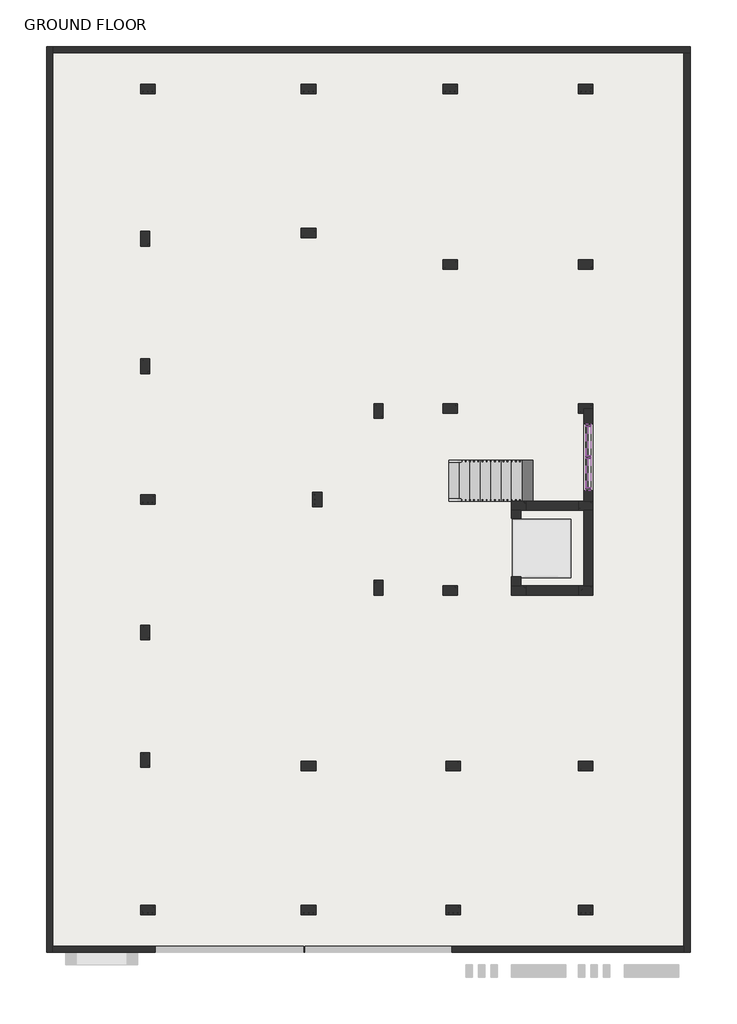
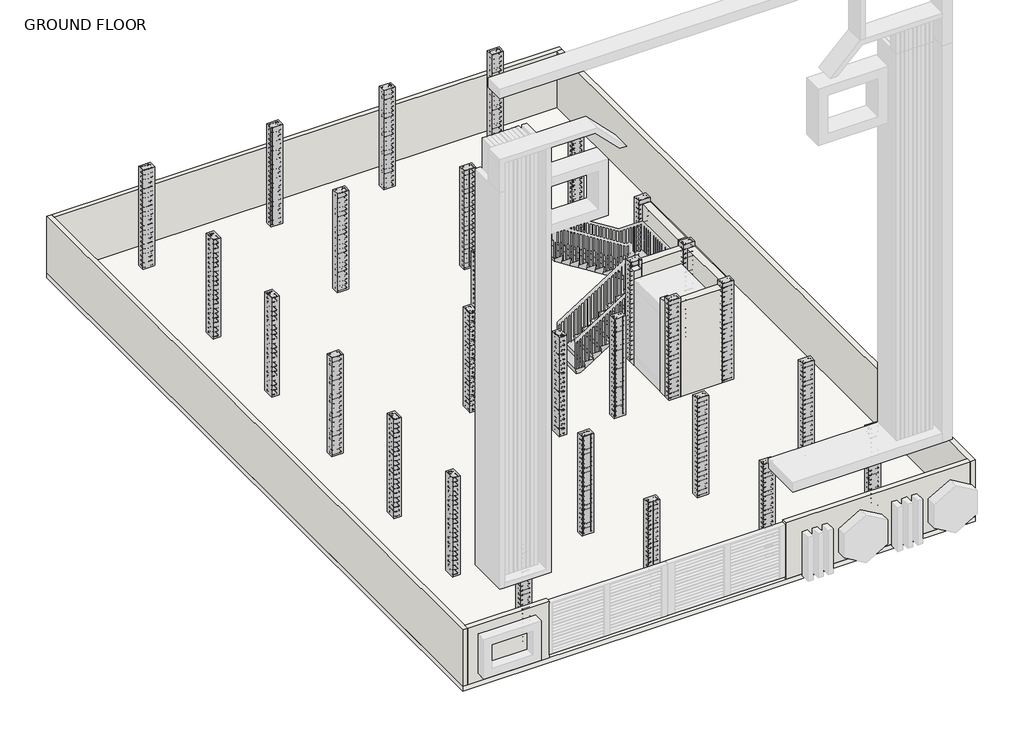
# One storey, part 1 of 7: 29 columns, 12 members, 12 walls, 4 plates, 1 slab, 1 stair flight.
"""IFC4 building model written with IfcOpenShell, lengths in millimetres."""

from ifc_helpers import new_model, si_unit, frame, origin, origin_with_axes, place, context, project, spatial, polyline, outline, extrude, faceted_brep, transform, mapped, element, save
from components import column_add0f710, member_7007ad49, member_abeaf8ac, member_a715cb85, member_410c6227, member_c4de40ee, member_73c23c35, system_panel_glazed_a527b3ca, system_panel_glazed_0825baf2

model = new_model("IFC4")

# Units and contexts
model_context = context("Model", 3, world=origin())
ifc_project = project(units=[si_unit("LENGTHUNIT", "METRE", prefix="MILLI")], contexts=[model_context])

# Site, building, storey
site = spatial("IfcSite", under=ifc_project)
building = spatial("IfcBuilding", under=site)
storey = spatial("IfcBuildingStorey", under=building, Name="GROUND FLOOR", Elevation=0.0)

# Columns
placement = place(None, origin())
column_shape = column_add0f710(model_context)
element("IfcColumn", 1, ObjectType="Concrete-Rectangular-Column : 1'2\"X9\"", at=placement, inside=storey, context=model_context, shape_type="MappedRepresentation", body=[
    mapped(column_shape, transform((-6074.3833787, 10029.759934, 0.0), x_axis=(0.0, 1.0, 0.0), y_axis=(-1.0, 0.0, 0.0), z_axis=(0.0, 0.0, 1.0))),
])
element("IfcColumn", 2, ObjectType="Concrete-Rectangular-Column : 1'2\"X9\"", at=placement, inside=storey, context=model_context, shape_type="MappedRepresentation", body=[
    mapped(column_shape, transform((-2162.7833787, 10029.759934, 0.0), x_axis=(0.0, 1.0, 0.0), y_axis=(-1.0, 0.0, 0.0), z_axis=(0.0, 0.0, 1.0))),
])
element("IfcColumn", 3, ObjectType="Concrete-Rectangular-Column : 1'2\"X9\"", at=placement, inside=storey, context=model_context, shape_type="MappedRepresentation", body=[
    mapped(column_shape, transform((1278.9166213, 10029.759934, 0.0), x_axis=(0.0, 1.0, 0.0), y_axis=(-1.0, 0.0, 0.0), z_axis=(0.0, 0.0, 1.0))),
])
element("IfcColumn", 4, ObjectType="Concrete-Rectangular-Column : 1'2\"X9\"", at=placement, inside=storey, context=model_context, shape_type="MappedRepresentation", body=[
    mapped(column_shape, transform((4580.9166213, 10029.759934, 0.0), x_axis=(0.0, 1.0, 0.0), y_axis=(-1.0, 0.0, 0.0), z_axis=(0.0, 0.0, 1.0))),
])
element("IfcColumn", 5, ObjectType="Concrete-Rectangular-Column : 1'2\"X9\"", at=placement, inside=storey, context=model_context, shape_type="MappedRepresentation", body=[
    mapped(column_shape, transform((4580.9166213, 5762.559934, 0.0), x_axis=(0.0, 1.0, 0.0), y_axis=(-1.0, 0.0, 0.0), z_axis=(0.0, 0.0, 1.0))),
])
element("IfcColumn", 6, ObjectType="Concrete-Rectangular-Column : 1'2\"X9\"", at=placement, inside=storey, context=model_context, shape_type="MappedRepresentation", body=[
    mapped(column_shape, transform((1278.9166213, 5762.559934, 0.0), x_axis=(0.0, 1.0, 0.0), y_axis=(-1.0, 0.0, 0.0), z_axis=(0.0, 0.0, 1.0))),
])
element("IfcColumn", 7, ObjectType="Concrete-Rectangular-Column : 1'2\"X9\"", at=placement, inside=storey, context=model_context, shape_type="MappedRepresentation", body=[
    mapped(column_shape, transform((-2162.7833787, 6524.559934, 0.0), x_axis=(0.0, 1.0, 0.0), y_axis=(-1.0, 0.0, 0.0), z_axis=(0.0, 0.0, 1.0))),
])
element("IfcColumn", 8, ObjectType="Concrete-Rectangular-Column : 1'2\"X9\"", at=placement, inside=storey, context=model_context, shape_type="MappedRepresentation", body=[
    mapped(column_shape, transform((-6137.8833787, 6384.859934, 0.0), x_axis=(-1.0, 0.0, 0.0), y_axis=(0.0, -1.0, 0.0), z_axis=(0.0, 0.0, 1.0))),
])
element("IfcColumn", 9, ObjectType="Concrete-Rectangular-Column : 1'2\"X9\"", at=placement, inside=storey, context=model_context, shape_type="MappedRepresentation", body=[
    mapped(column_shape, transform((-6137.8833787, 3286.059934, 0.0), x_axis=(-1.0, 0.0, 0.0), y_axis=(0.0, -1.0, 0.0), z_axis=(0.0, 0.0, 1.0))),
])
element("IfcColumn", 10, ObjectType="Concrete-Rectangular-Column : 1'2\"X9\"", at=placement, inside=storey, context=model_context, shape_type="MappedRepresentation", body=[
    mapped(column_shape, transform((-460.9833787, 2193.859934, 0.0), x_axis=(-1.0, 0.0, 0.0), y_axis=(0.0, -1.0, 0.0), z_axis=(0.0, 0.0, 1.0))),
])
element("IfcColumn", 11, ObjectType="Concrete-Rectangular-Column : 1'2\"X9\"", at=placement, inside=storey, context=model_context, shape_type="MappedRepresentation", body=[
    mapped(column_shape, transform((1278.9166213, 2257.359934, 0.0), x_axis=(0.0, -1.0, 0.0), y_axis=(1.0, 0.0, 0.0), z_axis=(0.0, 0.0, 1.0))),
])
element("IfcColumn", 12, ObjectType="Concrete-Rectangular-Column : 1'2\"X9\"", at=placement, inside=storey, context=model_context, shape_type="MappedRepresentation", body=[
    mapped(column_shape, transform((4580.9166213, 2257.359934, 0.0), x_axis=(0.0, -1.0, 0.0), y_axis=(1.0, 0.0, 0.0), z_axis=(0.0, 0.0, 1.0))),
])
element("IfcColumn", 13, ObjectType="Concrete-Rectangular-Column : 1'2\"X9\"", at=placement, inside=storey, context=model_context, shape_type="MappedRepresentation", body=[
    mapped(column_shape, transform((4580.9166213, -104.840066, 0.0), x_axis=(0.0, -1.0, 0.0), y_axis=(1.0, 0.0, 0.0), z_axis=(0.0, 0.0, 1.0))),
])
element("IfcColumn", 14, ObjectType="Concrete-Rectangular-Column : 1'2\"X9\"", at=placement, inside=storey, context=model_context, shape_type="MappedRepresentation", body=[
    mapped(column_shape, transform((2955.3166213, -104.840066, 0.0), x_axis=(0.0, -1.0, 0.0), y_axis=(1.0, 0.0, 0.0), z_axis=(0.0, 0.0, 1.0))),
])
element("IfcColumn", 15, ObjectType="Concrete-Rectangular-Column : 1'2\"X9\"", at=placement, inside=storey, context=model_context, shape_type="MappedRepresentation", body=[
    mapped(column_shape, transform((-1946.8833787, 47.559934, 0.0), x_axis=(1.0, 0.0, 0.0), y_axis=(0.0, 1.0, 0.0), z_axis=(0.0, 0.0, 1.0))),
])
element("IfcColumn", 16, ObjectType="Concrete-Rectangular-Column : 1'2\"X9\"", at=placement, inside=storey, context=model_context, shape_type="MappedRepresentation", body=[
    mapped(column_shape, transform((-6074.3833787, 47.559934, 0.0), x_axis=(0.0, 1.0, 0.0), y_axis=(-1.0, 0.0, 0.0), z_axis=(0.0, 0.0, 1.0))),
])
element("IfcColumn", 17, ObjectType="Concrete-Rectangular-Column : 1'2\"X9\"", at=placement, inside=storey, context=model_context, shape_type="MappedRepresentation", body=[
    mapped(column_shape, transform((-6137.8833787, -3190.940066, 0.0), x_axis=(-1.0, 0.0, 0.0), y_axis=(0.0, -1.0, 0.0), z_axis=(0.0, 0.0, 1.0))),
])
element("IfcColumn", 18, ObjectType="Concrete-Rectangular-Column : 1'2\"X9\"", at=placement, inside=storey, context=model_context, shape_type="MappedRepresentation", body=[
    mapped(column_shape, transform((-6137.8833787, -6289.740066, 0.0), x_axis=(-1.0, 0.0, 0.0), y_axis=(0.0, -1.0, 0.0), z_axis=(0.0, 0.0, 1.0))),
])
element("IfcColumn", 19, ObjectType="Concrete-Rectangular-Column : 1'2\"X9\"", at=placement, inside=storey, context=model_context, shape_type="MappedRepresentation", body=[
    mapped(column_shape, transform((-2162.7833787, -6429.440066, 0.0), x_axis=(0.0, -1.0, 0.0), y_axis=(1.0, 0.0, 0.0), z_axis=(0.0, 0.0, 1.0))),
])
element("IfcColumn", 20, ObjectType="Concrete-Rectangular-Column : 1'2\"X9\"", at=placement, inside=storey, context=model_context, shape_type="MappedRepresentation", body=[
    mapped(column_shape, transform((-6074.3833787, -9934.640066, 0.0), x_axis=(0.0, -1.0, 0.0), y_axis=(1.0, 0.0, 0.0), z_axis=(0.0, 0.0, 1.0))),
])
element("IfcColumn", 21, ObjectType="Concrete-Rectangular-Column : 1'2\"X9\"", at=placement, inside=storey, context=model_context, shape_type="MappedRepresentation", body=[
    mapped(column_shape, transform((-2162.7833787, -9934.640066, 0.0), x_axis=(0.0, -1.0, 0.0), y_axis=(1.0, 0.0, 0.0), z_axis=(0.0, 0.0, 1.0))),
])
element("IfcColumn", 22, ObjectType="Concrete-Rectangular-Column : 1'2\"X9\"", at=placement, inside=storey, context=model_context, shape_type="MappedRepresentation", body=[
    mapped(column_shape, transform((1355.1166213, -9934.640066, 0.0), x_axis=(0.0, -1.0, 0.0), y_axis=(1.0, 0.0, 0.0), z_axis=(0.0, 0.0, 1.0))),
])
element("IfcColumn", 23, ObjectType="Concrete-Rectangular-Column : 1'2\"X9\"", at=placement, inside=storey, context=model_context, shape_type="MappedRepresentation", body=[
    mapped(column_shape, transform((4580.9166213, -9934.640066, 0.0), x_axis=(0.0, -1.0, 0.0), y_axis=(1.0, 0.0, 0.0), z_axis=(0.0, 0.0, 1.0))),
])
element("IfcColumn", 24, ObjectType="Concrete-Rectangular-Column : 1'2\"X9\"", at=placement, inside=storey, context=model_context, shape_type="MappedRepresentation", body=[
    mapped(column_shape, transform((4580.9166213, -6429.440066, 0.0), x_axis=(0.0, -1.0, 0.0), y_axis=(1.0, 0.0, 0.0), z_axis=(0.0, 0.0, 1.0))),
])
element("IfcColumn", 25, ObjectType="Concrete-Rectangular-Column : 1'2\"X9\"", at=placement, inside=storey, context=model_context, shape_type="MappedRepresentation", body=[
    mapped(column_shape, transform((1355.1166213, -6429.440066, 0.0), x_axis=(0.0, -1.0, 0.0), y_axis=(1.0, 0.0, 0.0), z_axis=(0.0, 0.0, 1.0))),
])
element("IfcColumn", 26, ObjectType="Concrete-Rectangular-Column : 1'2\"X9\"", at=placement, inside=storey, context=model_context, shape_type="MappedRepresentation", body=[
    mapped(column_shape, transform((1278.9166213, -2162.240066, 0.0), x_axis=(0.0, -1.0, 0.0), y_axis=(1.0, 0.0, 0.0), z_axis=(0.0, 0.0, 1.0))),
])
element("IfcColumn", 27, ObjectType="Concrete-Rectangular-Column : 1'2\"X9\"", at=placement, inside=storey, context=model_context, shape_type="MappedRepresentation", body=[
    mapped(column_shape, transform((2955.3166213, -2162.240066, 0.0), x_axis=(0.0, -1.0, 0.0), y_axis=(1.0, 0.0, 0.0), z_axis=(0.0, 0.0, 1.0))),
])
element("IfcColumn", 28, ObjectType="Concrete-Rectangular-Column : 1'2\"X9\"", at=placement, inside=storey, context=model_context, shape_type="MappedRepresentation", body=[
    mapped(column_shape, transform((4580.9166213, -2162.240066, 0.0), x_axis=(0.0, -1.0, 0.0), y_axis=(1.0, 0.0, 0.0), z_axis=(0.0, 0.0, 1.0))),
])
element("IfcColumn", 29, ObjectType="Concrete-Rectangular-Column : 1'2\"X9\"", at=placement, inside=storey, context=model_context, shape_type="MappedRepresentation", body=[
    mapped(column_shape, transform((-460.9833787, -2098.740066, 0.0), x_axis=(1.0, 0.0, 0.0), y_axis=(0.0, 1.0, 0.0), z_axis=(0.0, 0.0, 1.0))),
])

# Members
member_shape = member_7007ad49(model_context)
element("IfcMember", 30, ObjectType="Rectangular Mullion : 2.5\" x 5\" rectangular", at=placement, inside=storey, context=model_context, shape_type="MappedRepresentation", body=[
    mapped(member_shape, transform((4644.4166213, 1825.559934, 2438.4), x_axis=(0.0, 0.0, 1.0), y_axis=(1.0, 0.0, 0.0), z_axis=(0.0, 1.0, 0.0))),
])
element("IfcMember", 31, ObjectType="Rectangular Mullion : 2.5\" x 5\" rectangular", at=placement, inside=storey, context=model_context, shape_type="MappedRepresentation", body=[
    mapped(member_shape, transform((4644.4166213, 1044.509934, 2438.4), x_axis=(0.0, 0.0, 1.0), y_axis=(1.0, 0.0, 0.0), z_axis=(0.0, 1.0, 0.0))),
])
element("IfcMember", 32, ObjectType="Rectangular Mullion : 2.5\" x 5\" rectangular", at=placement, inside=storey, context=model_context, shape_type="MappedRepresentation", body=[
    mapped(member_shape, transform((4644.4166213, 326.959934, 457.2), x_axis=(0.0, 0.0, -1.0), y_axis=(1.0, 0.0, 0.0), z_axis=(0.0, -1.0, 0.0))),
])
element("IfcMember", 33, ObjectType="Rectangular Mullion : 2.5\" x 5\" rectangular", at=placement, inside=storey, context=model_context, shape_type="MappedRepresentation", body=[
    mapped(member_shape, transform((4644.4166213, 1108.009934, 457.2), x_axis=(0.0, 0.0, -1.0), y_axis=(1.0, 0.0, 0.0), z_axis=(0.0, -1.0, 0.0))),
])
member_2_shape = member_abeaf8ac(model_context)
element("IfcMember", 34, ObjectType="Rectangular Mullion : 2.5\" x 5\" rectangular", at=placement, inside=storey, context=model_context, shape_type="MappedRepresentation", body=[
    mapped(member_2_shape, transform((4644.4166213, 1044.509934, 1524.0), x_axis=(0.0, 0.0, 1.0), y_axis=(1.0, 0.0, 0.0), z_axis=(0.0, 1.0, 0.0))),
])
element("IfcMember", 35, ObjectType="Rectangular Mullion : 2.5\" x 5\" rectangular", at=placement, inside=storey, context=model_context, shape_type="MappedRepresentation", body=[
    mapped(member_2_shape, transform((4644.4166213, 1825.559934, 1524.0), x_axis=(0.0, 0.0, 1.0), y_axis=(1.0, 0.0, 0.0), z_axis=(0.0, 1.0, 0.0))),
])
member_3_shape = member_a715cb85(model_context)
element("IfcMember", 36, ObjectType="Rectangular Mullion : 2.5\" x 5\" rectangular", at=placement, inside=storey, context=model_context, shape_type="MappedRepresentation", body=[
    mapped(member_3_shape, transform((4644.4166213, 1076.259934, 457.2), x_axis=(0.0, 1.0, 0.0), y_axis=(1.0, 0.0, 0.0), z_axis=(0.0, 0.0, -1.0))),
])
member_4_shape = member_410c6227(model_context)
element("IfcMember", 37, ObjectType="Rectangular Mullion : 2.5\" x 5\" rectangular", at=placement, inside=storey, context=model_context, shape_type="MappedRepresentation", body=[
    mapped(member_4_shape, transform((4644.4166213, 1076.259934, 1524.0), x_axis=(0.0, 1.0, 0.0), y_axis=(1.0, 0.0, 0.0), z_axis=(0.0, 0.0, -1.0))),
])
member_5_shape = member_c4de40ee(model_context)
element("IfcMember", 38, ObjectType="Rectangular Mullion : 2.5\" x 5\" rectangular", at=placement, inside=storey, context=model_context, shape_type="MappedRepresentation", body=[
    mapped(member_5_shape, transform((4644.4166213, 1889.059934, 457.2), x_axis=(0.0, 1.0, 0.0), y_axis=(1.0, 0.0, 0.0), z_axis=(0.0, 0.0, -1.0))),
])
member_6_shape = member_73c23c35(model_context)
element("IfcMember", 39, ObjectType="Rectangular Mullion : 2.5\" x 5\" rectangular", at=placement, inside=storey, context=model_context, shape_type="MappedRepresentation", body=[
    mapped(member_6_shape, transform((4644.4166213, 263.459934, 2438.4), x_axis=(0.0, -1.0, 0.0), y_axis=(1.0, 0.0, 0.0), z_axis=(0.0, 0.0, 1.0))),
])
element("IfcMember", 40, ObjectType="Rectangular Mullion : 2.5\" x 5\" rectangular", at=placement, inside=storey, context=model_context, shape_type="MappedRepresentation", body=[
    mapped(member_6_shape, transform((4644.4166213, 1889.059934, 1524.0), x_axis=(0.0, 1.0, 0.0), y_axis=(1.0, 0.0, 0.0), z_axis=(0.0, 0.0, -1.0))),
])
element("IfcMember", 41, ObjectType="Rectangular Mullion : 2.5\" x 5\" rectangular", at=placement, inside=storey, context=model_context, shape_type="MappedRepresentation", body=[
    mapped(member_5_shape, transform((4644.4166213, 263.459934, 1524.0), x_axis=(0.0, -1.0, 0.0), y_axis=(1.0, 0.0, 0.0), z_axis=(0.0, 0.0, 1.0))),
])

# Plates
system_panel_glazed_shape = system_panel_glazed_a527b3ca(model_context)
element("IfcPlate", 42, ObjectType="System Panel : Glazed", at=placement, inside=storey, context=model_context, shape_type="MappedRepresentation", body=[
    mapped(system_panel_glazed_shape, transform((4644.4166213, 685.734934, 520.7), x_axis=(0.0, 1.0, 0.0), y_axis=(-1.0, 0.0, 0.0), z_axis=(0.0, 0.0, 1.0))),
])
element("IfcPlate", 43, ObjectType="System Panel : Glazed", at=placement, inside=storey, context=model_context, shape_type="MappedRepresentation", body=[
    mapped(system_panel_glazed_shape, transform((4644.4166213, 1466.784934, 520.7), x_axis=(0.0, 1.0, 0.0), y_axis=(-1.0, 0.0, 0.0), z_axis=(0.0, 0.0, 1.0))),
])
system_panel_glazed_2_shape = system_panel_glazed_0825baf2(model_context)
element("IfcPlate", 44, ObjectType="System Panel : Glazed", at=placement, inside=storey, context=model_context, shape_type="MappedRepresentation", body=[
    mapped(system_panel_glazed_2_shape, transform((4644.4166213, 685.734934, 1555.75), x_axis=(0.0, 1.0, 0.0), y_axis=(-1.0, 0.0, 0.0), z_axis=(0.0, 0.0, 1.0))),
])
element("IfcPlate", 45, ObjectType="System Panel : Glazed", at=placement, inside=storey, context=model_context, shape_type="MappedRepresentation", body=[
    mapped(system_panel_glazed_2_shape, transform((4644.4166213, 1466.784934, 1555.75), x_axis=(0.0, 1.0, 0.0), y_axis=(-1.0, 0.0, 0.0), z_axis=(0.0, 0.0, 1.0))),
])

# Slab
element("IfcSlab", 46, ObjectType="6\"", at=placement, inside=storey, context=model_context, shape_type="SweptSolid", body=[
    extrude(outline(polyline([(7120.9166213, 11058.459934), (7120.9166213, -10963.340066), (-8538.1833787, -10963.340066), (-8538.1833787, 11058.459934), (7120.9166213, 11058.459934)])), frame((0.0, 0.0, -152.4), z_axis=(0.0, 0.0, 1.0), x_axis=(1.0, 0.0, 0.0)), (0.0, 0.0, 1.0), 152.4),
])

# Stair flight
element("IfcStairFlight", 47, ObjectType="3/4\" Nosing", at=placement, inside=storey, context=model_context, shape_type="Brep", body=[
    faceted_brep([(1253.5166213, 9.459934, 160.02), (1253.5166213, 1000.059934, 160.02), (1272.5666213, 1000.059934, 0.0), (1272.5666213, 9.459934, 0.0), (1526.5666213, 9.459934, 160.02), (1526.5666213, 1000.059934, 160.02), (1526.5666213, 1000.059934, 84.9690172), (1391.6951655, 1000.059934, 0.0), (1391.6951655, 9.459934, 0.0), (1526.5666213, 9.459934, 84.9690172), (1507.5166213, 1000.059934, 320.04), (1507.5166213, 9.459934, 320.04), (1780.5666213, 9.459934, 320.04), (1780.5666213, 1000.059934, 320.04), (1780.5666213, 1000.059934, 244.9890172), (1780.5666213, 9.459934, 244.9890172), (1761.5166213, 1000.059934, 480.06), (1761.5166213, 9.459934, 480.06), (2034.5666213, 9.459934, 480.06), (2034.5666213, 1000.059934, 480.06), (2034.5666213, 1000.059934, 405.0090172), (2034.5666213, 9.459934, 405.0090172), (2015.5166213, 1000.059934, 640.08), (2015.5166213, 9.459934, 640.08), (2288.5666213, 9.459934, 640.08), (2288.5666213, 1000.059934, 640.08), (2288.5666213, 1000.059934, 565.0290172), (2288.5666213, 9.459934, 565.0290172), (2269.5166213, 1000.059934, 800.1), (2269.5166213, 9.459934, 800.1), (2542.5666213, 9.459934, 800.1), (2542.5666213, 1000.059934, 800.1), (2542.5666213, 1000.059934, 725.0490172), (2542.5666213, 9.459934, 725.0490172), (2523.5166213, 1000.059934, 960.12), (2523.5166213, 9.459934, 960.12), (2796.5666213, 9.459934, 960.12), (2796.5666213, 1000.059934, 960.12), (2796.5666213, 1000.059934, 885.0690172), (2796.5666213, 9.459934, 885.0690172), (2777.5166213, 1000.059934, 1120.14), (2777.5166213, 9.459934, 1120.14), (3050.5666213, 9.459934, 1120.14), (3050.5666213, 1000.059934, 1120.14), (3050.5666213, 1000.059934, 1045.0890172), (3050.5666213, 9.459934, 1045.0890172), (3031.5166213, 1000.059934, 1280.16), (3031.5166213, 9.459934, 1280.16), (3304.5666213, 9.459934, 1280.16), (3304.5666213, 1000.059934, 1280.16), (3304.5666213, 1000.059934, 1205.1090172), (3304.5666213, 9.459934, 1205.1090172), (3558.5666213, 1000.059934, 1440.18), (3285.5166213, 1000.059934, 1440.18), (3285.5166213, 9.459934, 1440.18), (3558.5666213, 9.459934, 1440.18), (3547.0761451, 1000.059934, 1536.7), (3830.9015147, 1000.059934, 1536.7), (3558.5666213, 9.459934, 1365.1290172), (3520.4666213, 1152.459934, 1600.2), (3539.5166213, 1152.459934, 1600.2), (3539.5166213, 1000.059934, 1600.2), (3539.5166213, 9.459934, 1600.2), (3830.9015147, 9.459934, 1600.2), (4530.1166213, 9.459934, 1600.2), (4530.1166213, 2143.059934, 1600.2), (3520.4666213, 2143.059934, 1600.2), (3520.4666213, 1152.459934, 1536.7), (3539.5166213, 1152.459934, 1536.7), (3539.5166213, 1000.059934, 1536.7), (3830.9015147, 9.459934, 1536.7), (4530.1166213, 9.459934, 1536.7), (4530.1166213, 2143.059934, 1536.7), (3520.4666213, 2143.059934, 1536.7), (3539.5166213, 1152.459934, 1760.22), (3539.5166213, 2143.059934, 1760.22), (3502.1317279, 2143.059934, 1760.22), (3266.4666213, 2143.059934, 1760.22), (3266.4666213, 1152.459934, 1760.22), (3502.1317279, 1152.459934, 1760.22), (3266.4666213, 1152.459934, 1685.1690172), (3502.1317279, 1152.459934, 1536.7), (3502.1317279, 2143.059934, 1536.7), (3266.4666213, 2143.059934, 1685.1690172), (3285.5166213, 1152.459934, 1920.24), (3285.5166213, 2143.059934, 1920.24), (3012.4666213, 2143.059934, 1920.24), (3012.4666213, 1152.459934, 1920.24), (3012.4666213, 1152.459934, 1845.1890172), (3012.4666213, 2143.059934, 1845.1890172), (3031.5166213, 1152.459934, 2080.26), (3031.5166213, 2143.059934, 2080.26), (2758.4666213, 2143.059934, 2080.26), (2758.4666213, 1152.459934, 2080.26), (2758.4666213, 1152.459934, 2005.2090172), (2758.4666213, 2143.059934, 2005.2090172), (2777.5166213, 1152.459934, 2240.28), (2777.5166213, 2143.059934, 2240.28), (2504.4666213, 2143.059934, 2240.28), (2504.4666213, 1152.459934, 2240.28), (2504.4666213, 1152.459934, 2165.2290172), (2504.4666213, 2143.059934, 2165.2290172), (2523.5166213, 1152.459934, 2400.3), (2523.5166213, 2143.059934, 2400.3), (2250.4666213, 2143.059934, 2400.3), (2250.4666213, 1152.459934, 2400.3), (2250.4666213, 1152.459934, 2325.2490172), (2250.4666213, 2143.059934, 2325.2490172), (2269.5166213, 1152.459934, 2560.32), (2269.5166213, 2143.059934, 2560.32), (1996.4666213, 2143.059934, 2560.32), (1996.4666213, 1152.459934, 2560.32), (1996.4666213, 1152.459934, 2485.2690172), (1996.4666213, 2143.059934, 2485.2690172), (2015.5166213, 1152.459934, 2720.34), (2015.5166213, 2143.059934, 2720.34), (1742.4666213, 2143.059934, 2720.34), (1742.4666213, 1152.459934, 2720.34), (1742.4666213, 1152.459934, 2645.2890172), (1742.4666213, 2143.059934, 2645.2890172), (1761.5166213, 1152.459934, 2880.36), (1761.5166213, 2143.059934, 2880.36), (1488.4666213, 2143.059934, 2880.36), (1488.4666213, 1152.459934, 2880.36), (1488.4666213, 1152.459934, 2805.3090172), (1488.4666213, 2143.059934, 2805.3090172), (1507.5166213, 1152.459934, 3040.38), (1507.5166213, 2143.059934, 3040.38), (1253.5166213, 2143.059934, 3040.38), (1253.5166213, 1152.459934, 3040.38), (1253.5166213, 1152.459934, 2953.3275172), (1253.5166213, 2143.059934, 2953.3275172)], [[[0, 1, 2, 3]], [[1, 0, 4, 5]], [[1, 5, 6, 7, 2]], [[4, 0, 3, 8, 9]], [[10, 11, 12, 13]], [[10, 13, 14, 6, 5]], [[12, 11, 4, 9, 15]], [[5, 4, 11, 10]], [[16, 17, 18, 19]], [[16, 19, 20, 14, 13]], [[18, 17, 12, 15, 21]], [[13, 12, 17, 16]], [[22, 23, 24, 25]], [[22, 25, 26, 20, 19]], [[24, 23, 18, 21, 27]], [[19, 18, 23, 22]], [[28, 29, 30, 31]], [[28, 31, 32, 26, 25]], [[30, 29, 24, 27, 33]], [[25, 24, 29, 28]], [[34, 35, 36, 37]], [[34, 37, 38, 32, 31]], [[36, 35, 30, 33, 39]], [[31, 30, 35, 34]], [[40, 41, 42, 43]], [[40, 43, 44, 38, 37]], [[42, 41, 36, 39, 45]], [[37, 36, 41, 40]], [[46, 47, 48, 49]], [[46, 49, 50, 44, 43]], [[48, 47, 42, 45, 51]], [[43, 42, 47, 46]], [[52, 53, 54, 55]], [[52, 56, 57, 50, 49, 53]], [[55, 54, 48, 51, 58]], [[49, 48, 54, 53]], [[59, 60, 61, 62, 63, 64, 65, 66]], [[60, 59, 67, 68]], [[61, 60, 68, 69]], [[56, 61, 69]], [[62, 55, 58, 70, 71, 64, 63]], [[65, 64, 71, 72]], [[66, 65, 72, 73]], [[52, 55, 62, 61, 56]], [[74, 75, 76, 77, 78, 79]], [[59, 74, 79, 78, 80, 81, 67]], [[75, 66, 73, 82, 83, 77, 76]], [[59, 66, 75, 74]], [[84, 85, 86, 87]], [[84, 87, 88, 80, 78]], [[86, 85, 77, 83, 89]], [[78, 77, 85, 84]], [[90, 91, 92, 93]], [[90, 93, 94, 88, 87]], [[92, 91, 86, 89, 95]], [[87, 86, 91, 90]], [[96, 97, 98, 99]], [[96, 99, 100, 94, 93]], [[98, 97, 92, 95, 101]], [[93, 92, 97, 96]], [[102, 103, 104, 105]], [[102, 105, 106, 100, 99]], [[104, 103, 98, 101, 107]], [[99, 98, 103, 102]], [[108, 109, 110, 111]], [[108, 111, 112, 106, 105]], [[110, 109, 104, 107, 113]], [[105, 104, 109, 108]], [[114, 115, 116, 117]], [[114, 117, 118, 112, 111]], [[116, 115, 110, 113, 119]], [[111, 110, 115, 114]], [[120, 121, 122, 123]], [[120, 123, 124, 118, 117]], [[122, 121, 116, 119, 125]], [[117, 116, 121, 120]], [[126, 127, 128, 129]], [[126, 129, 130, 124, 123]], [[128, 127, 122, 125, 131]], [[129, 128, 131, 130]], [[123, 122, 127, 126]], [[3, 2, 7, 8]], [[50, 57, 70, 58, 51, 45, 39, 33, 27, 21, 15, 9, 8, 7, 6, 14, 20, 26, 32, 38, 44]], [[70, 57, 56, 69, 68, 67, 81, 82, 73, 72, 71]], [[82, 81, 80, 88, 94, 100, 106, 112, 118, 124, 130, 131, 125, 119, 113, 107, 101, 95, 89, 83]]]),
])

# Walls
element("IfcWall", 48, ObjectType="6\"", at=placement, inside=storey, context=model_context, shape_type="Brep", body=[
    faceted_brep([(-8538.1833787, 11058.459934, 0.0), (-8538.1833787, -10963.340066, 0.0), (-8538.1833787, -10963.340066, 1828.8), (-8538.1833787, 11058.459934, 1828.8), (-8385.7833787, 11058.459934, 0.0), (-8385.7833787, 11058.459934, 1828.8), (-8385.7833787, 10906.059934, 1828.8), (-8385.7833787, -10810.940066, 1828.8), (-8385.7833787, -10963.340066, 1828.8), (-8385.7833787, -10963.340066, 0.0), (-8385.7833787, -10810.940066, 0.0), (-8385.7833787, 10906.059934, 0.0)], [[[0, 1, 2, 3]], [[4, 5, 6, 7, 8, 9, 10, 11]], [[1, 0, 4, 11, 10, 9]], [[3, 2, 8, 7, 6, 5]], [[0, 3, 5, 4]], [[2, 1, 9, 8]]]),
])
element("IfcWall", 49, ObjectType="6\"", at=placement, inside=storey, context=model_context, shape_type="Brep", body=[
    faceted_brep([(-8385.7833787, 10906.059934, 0.0), (6968.5166213, 10906.059934, 0.0), (7120.9166213, 10906.059934, 0.0), (7120.9166213, 10906.059934, 1828.8), (6968.5166213, 10906.059934, 1828.8), (-8385.7833787, 10906.059934, 1828.8), (-8385.7833787, 11058.459934, 0.0), (-8385.7833787, 11058.459934, 1828.8), (7120.9166213, 11058.459934, 1828.8), (7120.9166213, 11058.459934, 0.0)], [[[0, 1, 2, 3, 4, 5]], [[6, 7, 8, 9]], [[2, 1, 0, 6, 9]], [[5, 4, 3, 8, 7]], [[0, 5, 7, 6]], [[3, 2, 9, 8]]]),
])
element("IfcWall", 50, ObjectType="6\"", at=placement, inside=storey, context=model_context, shape_type="Brep", body=[
    faceted_brep([(6968.5166213, 10906.059934, 0.0), (6968.5166213, -10810.940066, 0.0), (6968.5166213, -10963.340066, 0.0), (6968.5166213, -10963.340066, 1828.8), (6968.5166213, -10810.940066, 1828.8), (6968.5166213, 10906.059934, 1828.8), (7120.9166213, 10906.059934, 0.0), (7120.9166213, 10906.059934, 1828.8), (7120.9166213, -10963.340066, 1828.8), (7120.9166213, -10963.340066, 0.0)], [[[0, 1, 2, 3, 4, 5]], [[6, 7, 8, 9]], [[2, 1, 0, 6, 9]], [[5, 4, 3, 8, 7]], [[0, 5, 7, 6]], [[3, 2, 9, 8]]]),
])
element("IfcWall", 51, ObjectType="6\"", at=placement, inside=storey, context=model_context, shape_type="SweptSolid", body=[
    extrude(outline(polyline([(1329.7166213, -10810.940066), (6968.5166213, -10810.940066), (6968.5166213, -10963.340066), (1329.7166213, -10963.340066), (1329.7166213, -10810.940066)])), origin_with_axes(), (0.0, 0.0, 1.0), 1828.8),
])
element("IfcWall", 52, ObjectType="6\"", at=placement, inside=storey, context=model_context, shape_type="SweptSolid", body=[
    extrude(outline(polyline([(-5896.5833787, -10963.340066), (-8385.7833787, -10963.340066), (-8385.7833787, -10810.940066), (-5896.5833787, -10810.940066), (-5896.5833787, -10963.340066)])), origin_with_axes(), (0.0, 0.0, 1.0), 1828.8),
])
element("IfcWall", 53, ObjectType="9\"", at=placement, inside=storey, context=model_context, shape_type="SweptSolid", body=[
    extrude(outline(polyline([(3133.1166213, 9.459934), (4403.1166213, 9.459934), (4403.1166213, -219.140066), (3133.1166213, -219.140066), (3133.1166213, 9.459934)])), origin_with_axes(), (0.0, 0.0, 1.0), 3048.0),
])
element("IfcWall", 54, ObjectType="9\"", at=placement, inside=storey, context=model_context, shape_type="SweptSolid", body=[
    extrude(outline(polyline([(2777.5166213, -407.140066), (2777.5166213, -219.140066), (3006.1166213, -219.140066), (3006.1166213, -407.140066), (2777.5166213, -407.140066)])), origin_with_axes(), (0.0, 0.0, 1.0), 3048.0),
])
element("IfcWall", 55, ObjectType="9\"", at=placement, inside=storey, context=model_context, shape_type="SweptSolid", body=[
    extrude(outline(polyline([(2777.5166213, -2047.940066), (2777.5166213, -1831.140066), (3006.1166213, -1831.140066), (3006.1166213, -2047.940066), (2777.5166213, -2047.940066)])), origin_with_axes(), (0.0, 0.0, 1.0), 3048.0),
])
element("IfcWall", 56, ObjectType="9\"", at=placement, inside=storey, context=model_context, shape_type="SweptSolid", body=[
    extrude(outline(polyline([(4403.1166213, -2276.540066), (3133.1166213, -2276.540066), (3133.1166213, -2047.940066), (4403.1166213, -2047.940066), (4403.1166213, -2276.540066)])), origin_with_axes(), (0.0, 0.0, 1.0), 3048.0),
])
element("IfcWall", 57, ObjectType="9\"", at=placement, inside=storey, context=model_context, shape_type="SweptSolid", body=[
    extrude(outline(polyline([(4530.1166213, -2047.940066), (4530.1166213, -219.140066), (4758.7166213, -219.140066), (4758.7166213, -2047.940066), (4530.1166213, -2047.940066)])), origin_with_axes(), (0.0, 0.0, 1.0), 3048.0),
])
element("IfcWall", 58, ObjectType="9\"", at=placement, inside=storey, context=model_context, shape_type="SweptSolid", body=[
    extrude(outline(polyline([(4758.7166213, 263.459934), (4758.7166213, 9.459934), (4530.1166213, 9.459934), (4530.1166213, 263.459934), (4758.7166213, 263.459934)])), origin_with_axes(), (0.0, 0.0, 1.0), 3048.0),
])
element("IfcWall", 59, ObjectType="9\"", at=placement, inside=storey, context=model_context, shape_type="SweptSolid", body=[
    extrude(outline(polyline([(2257.359934, 0.0), (263.459934, 0.0), (263.459934, 457.2), (1889.059934, 457.2), (1889.059934, 2438.4), (263.459934, 2438.4), (263.459934, 3048.0), (2257.359934, 3048.0), (2257.359934, 0.0)])), frame((4530.1166213, 0.0, 0.0), z_axis=(1.0, 0.0, 0.0), x_axis=(0.0, 1.0, 0.0)), (0.0, 0.0, 1.0), 228.6),
])

save(model, "model.ifc")

# Revit data of these elements
# Type "Concrete-Rectangular-Column : 1'2\"X9\""
#   Assembly Code = "B10"
#   b = 0' - 9"
#   h = 1' - 2"
#   Structural Material [instance default] = Concrete, Cast-in-Place gray
# Type "Rectangular Mullion : 2.5\" x 5\" rectangular"
#   built-in parameter 1007304 = 0.416667 (stored number, unit not read)
#   built-in parameter 1007301 = 0.104167 (stored number, unit not read)
#   built-in parameter 1007300 = 0.104167 (stored number, unit not read)
# Type "System Panel : Glazed"
#   Construction Type Id = "GSP4R"
#   Analytic Construction = "1/8 in Pilkington single glazing"
#   Visual Light Transmittance = 0.9
#   Solar Heat Gain Coefficient = 0.86
#   Heat Transfer Coefficient (U) = 1.18115 BTU/(h·ft²·°F)
#   Define Thermal Properties by = 1
# Type "6\""
#   Assembly Code = "B1010"
#   Function = 0
#   Layers, outside or top first: 0' - 6" no material (function 1)
# Type "6\""
#   Assembly Code = "B2010"
#   Layers, outside or top first: 0' - 6" "6\" wall" (function 1)
# Type "9\""
#   Assembly Code = "B2010"
#   Layers, outside or top first: 0' - 9" "charcoal grey" (function 1)
# Elements 1, 2, 3, 4, 5, 6, 7, 8, 9, 10, 11, 12, 13, 14, 15, 16, 17, 18, 19, 20, 21, 22, 23, 24, 25, 26, 27, 28, 29 (IfcColumn, "Concrete-Rectangular-Column : 1'2\"X9\"")
#   Structural Material = Concrete, Cast-in-Place gray
#   Phase Created = New Construction
#   Materials on its faces: "Concrete, Cast-in-Place gray"
# Elements 30, 31, 32, 33, 34, 35, 36, 37, 38, 39, 40, 41 (IfcMember, "Rectangular Mullion : 2.5\" x 5\" rectangular")
#   Phase Created = New Construction
#   Materials on its faces: "Aluminum"
# Elements 42, 43, 44, 45 (IfcPlate, "System Panel : Glazed")
#   Phase Created = New Construction
#   Materials on its faces: "Glass"
# Element 46 (IfcSlab, "6\"")
#   Height Offset From Level = 0' - 0"
#   Phase Created = New Construction
#   Materials on its faces: "Default Floor"
# Element 47 (IfcStairFlight, "3/4\" Nosing")
#   Phase Created = New Construction
#   Materials on its faces: "Concrete, Cast-in-Place gray"
# Elements 48, 49, 50, 51, 52 (IfcWall, "6\"")
#   Top Offset = -0' - 6"
#   Base Offset = 0' - 0"
#   Unconnected Height = 6' - 0"
#   wall height = 6' - 0"
#   Phase Created = New Construction
#   Base Constraint = GROUND FLOOR
#   Materials on its faces: "6\" wall"
# Elements 53, 54, 55, 56, 57, 58, 59 (IfcWall, "9\"")
#   Top Offset = -0' - 6"
#   Base Offset = 0' - 0"
#   wall height = 10' - 0"
#   Phase Created = New Construction
#   Base Constraint = GROUND FLOOR
#   Top Constraint = FIRST FLOOR
#   Materials on its faces: "charcoal grey"
# Materials
#   "Concrete, Cast-in-Place gray": class "Concrete", colour RGB 192 192 192, transparency 0, Description = "Cast-in-place concrete", Cost = 0
#   "6\" wall": class "Generic", colour RGB 245 239 227, transparency 0, Cost = 0
#   "charcoal grey": class "Generic", colour RGB 54 69 79, transparency 0, Cost = 0
#   "Aluminum": class "Metal", colour RGB 247 247 247, transparency 0, Description = "Aluminum 6061", Cost = 0
#   "Glass": class "Glass", colour RGB 0 128 192, transparency 0.75, Description = "Soda Lime Glass", Cost = 0
#   "Default Floor": colour RGB 128 128 128, transparency 0, Cost = 0
